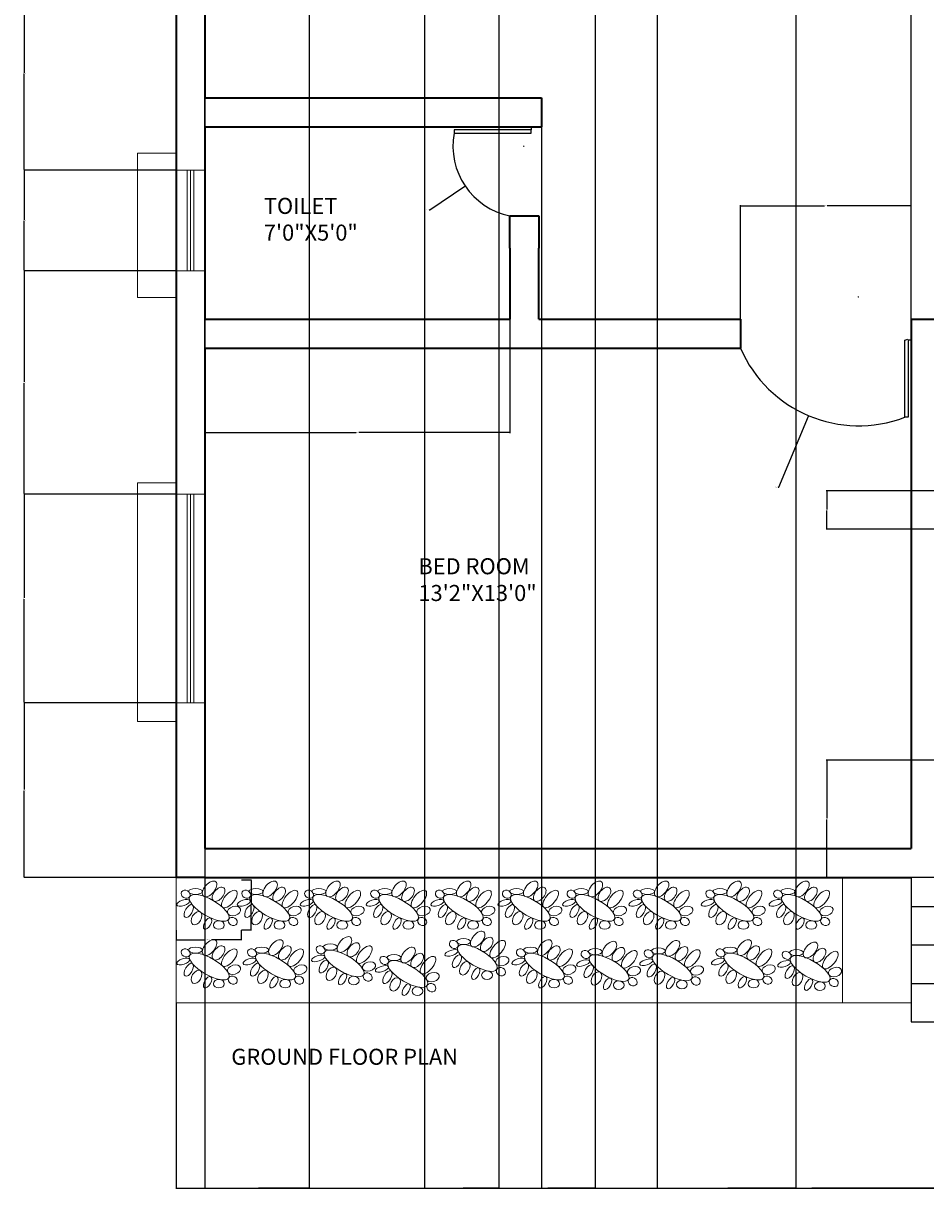
# Model space of a CAD drawing. Units: inches. Extents: x -35 to 633, y -653 to 119.
# Tile 1 of 4: x -35 to 246, y -653 to -289. Entities that reach past the tile are written whole.
import ezdxf

# ---------------------------------------------------------------- set-up
doc = ezdxf.new("R2010")
doc.units = ezdxf.units.IN
doc.header["$MEASUREMENT"] = 0
for name, color, linetype, lineweight in [('A-ANNO-DIMS', 2, 'Continuous', 18), ('A-ANNO-TEXT', 7, 'Continuous', 25), ('A-AREA-IDEN', 7, 'Continuous', 18), ('A-DOOR', 3, 'Continuous', 25), ('A-FLOR-STRS', 7, 'Continuous', 25), ('A-GLAZ', 4, 'Continuous', 20), ('A-GLAZ-PROJ', 4, 'Continuous', 18), ('A-WALL', 7, 'Continuous', 35), ('L-PLNT', 3, 'Continuous', 13), ('L-PLNT-BEDS', 94, 'Continuous', 20)]:
    doc.layers.add(name, color=color, linetype=linetype, lineweight=lineweight)
doc.styles.get("Standard").update_dxf_attribs({"font": 'arial.ttf'})
doc.dimstyles.get("Standard").update_dxf_attribs({"dimtxt": 0.18, "dimasz": 0.18, "dimexe": 0.18, "dimexo": 0.0625, "dimgap": 0.09, "dimtad": 0, "dimtih": 1, "dimtoh": 1, "dimdec": 4, "dimzin": 0, "dimdsep": 46, "dimtxsty": 'Standard', "dimcen": 0.09, "dimadec": 0, "dimazin": 0, "dimtfac": 1, "dimtdec": 4, "dimtofl": 0, "dimtmove": 0, "dimatfit": 3, "dimfxl": 1, "dimtolj": 1, "dimtzin": 0, "dimarcsym": 0})

# ---------------------------------------------------------------- blocks, each defined once
blk = doc.blocks.new('SHRUB-PLAN')
for centre, major_axis, ratio in [((0.11, 5.9), (-1.92, -2.24), 0.535049), ((-7.34, 4.24), (1.26, -0.73), 0.824136), ((0, 0), (-6.08, 3.51), 0.369459), ((-4.3, 5.11), (2.15, 0), 0.440675), ((2.91, 4.24), (-1.61, -2), 0.581787), ((6.3, 2.75), (-2.14, -2.56), 0.458164), ((-8.09, 1.57), (2.03, 0.66), 0.398765), ((-6.37, -0.99), (1.12, 1.93), 0.488989), ((7.75, -0.97), (-2.05, -0.58), 0.66194), ((-3.94, -3.23), (1.13, 1.96), 0.622261), ((-0.49, -4.89), (1, 1.73), 0.484407), ((7.35, -4.24), (-1.27, 0.73), 0.849112), ((3.02, -5.34), (-1.69, 0), 0.789987)]:
    blk.add_ellipse(centre, major_axis=major_axis, ratio=ratio)
blk = doc.blocks.new('DOOR-LEAF-24IN')
for p, q in [((-1, 24), (-2, 24)), ((-2, 24), (-2, 0)), ((-1, 0), (-1, 24)), ((-2, 0), (-1, 0)), ((0, 0), (-1, 0))]:
    blk.add_line(p, q)
blk = doc.blocks.new('*D8')
at = {"layer": 'A-ANNO-DIMS', "color": 0, "lineweight": -2, "transparency": 16777216}
for p, q in [((12.74, -572.14), (12.74, -575.29)), ((33.02, -572.14), (33.02, -575.29)), ((12.92, -575.11), (21.88, -575.11)), ((32.84, -575.11), (23.88, -575.11))]:
    blk.add_line(p, q, dxfattribs=at)
at = {"layer": 'A-ANNO-DIMS', "color": 0, "transparency": 16777216}
for points in [[(12.92, -575.08), (12.92, -575.14), (12.74, -575.11)], [(32.84, -575.08), (32.84, -575.14), (33.02, -575.11)]]:
    blk.add_solid(points, dxfattribs=at)
at = {"layer": 'Defpoints', "color": 0, "transparency": 16777216}
for p in [(12.74, -572.07), (33.02, -572.07), (33.02, -575.11)]:
    blk.add_point(p, dxfattribs=at)
at = {"layer": 'A-ANNO-DIMS', "color": 0, "transparency": 16777216, "insert": (22.88, -575.11), "char_height": 0.18, "attachment_point": 5}
blk.add_mtext('\\A1;SHRUB 20 TYP.', dxfattribs=at)
blk = doc.blocks.new('*D9')
at = {"layer": 'A-ANNO-DIMS', "color": 0, "lineweight": -2, "transparency": 16777216}
for p, q in [((33.08, -556.48), (36.24, -556.48)), ((36.06, -556.66), (36.06, -564.09)), ((36.06, -571.89), (36.06, -564.46)), ((33.08, -572.07), (36.24, -572.07))]:
    blk.add_line(p, q, dxfattribs=at)
at = {"layer": 'A-ANNO-DIMS', "color": 0, "transparency": 16777216}
for points in [[(36.03, -556.66), (36.09, -556.66), (36.06, -556.48)], [(36.03, -571.89), (36.09, -571.89), (36.06, -572.07)]]:
    blk.add_solid(points, dxfattribs=at)
at = {"layer": 'Defpoints', "color": 0, "transparency": 16777216}
for p in [(33.02, -556.48), (36.06, -556.48), (33.02, -572.07)]:
    blk.add_point(p, dxfattribs=at)
at = {"layer": 'A-ANNO-DIMS', "color": 0, "transparency": 16777216, "insert": (36.06, -564.28), "char_height": 0.18, "attachment_point": 5}
blk.add_mtext('\\A1;16 TYP.', dxfattribs=at)
blk = doc.blocks.new('*D10')
at = {"layer": 'A-ANNO-DIMS', "color": 0, "lineweight": -2, "transparency": 16777216}
for p, q in [((12.69, -594.87), (12.69, -652.72)), ((585.69, -595.88), (585.69, -652.72)), ((12.87, -652.54), (298.9, -652.54)), ((585.51, -652.54), (299.48, -652.54))]:
    blk.add_line(p, q, dxfattribs=at)
at = {"layer": 'A-ANNO-DIMS', "color": 0, "transparency": 16777216}
for points in [[(12.87, -652.51), (12.87, -652.57), (12.69, -652.54)], [(585.51, -652.51), (585.51, -652.57), (585.69, -652.54)]]:
    blk.add_solid(points, dxfattribs=at)
at = {"layer": 'Defpoints', "color": 0, "transparency": 16777216}
for p in [(12.69, -594.81), (585.69, -595.82), (585.69, -652.54)]:
    blk.add_point(p, dxfattribs=at)
at = {"layer": 'A-ANNO-DIMS', "color": 0, "transparency": 16777216, "insert": (299.19, -652.54), "char_height": 0.18, "attachment_point": 5}
blk.add_mtext('\\A1;573', dxfattribs=at)
blk = doc.blocks.new('*D14')
at = {"layer": 'A-ANNO-DIMS', "color": 0, "lineweight": -2, "transparency": 16777216}
for p, q in [((21.69, 17.22), (21.69, -652.72)), ((54.19, 17.22), (54.19, -652.72)), ((21.87, -652.54), (37.47, -652.54)), ((54.01, -652.54), (38.4, -652.54))]:
    blk.add_line(p, q, dxfattribs=at)
at = {"layer": 'A-ANNO-DIMS', "color": 0, "transparency": 16777216}
for points in [[(21.87, -652.51), (21.87, -652.57), (21.69, -652.54)], [(54.01, -652.51), (54.01, -652.57), (54.19, -652.54)]]:
    blk.add_solid(points, dxfattribs=at)
at = {"layer": 'Defpoints', "color": 0, "transparency": 16777216}
for p in [(21.69, 17.29), (54.19, 17.29), (54.19, -652.54)]:
    blk.add_point(p, dxfattribs=at)
at = {"layer": 'A-ANNO-DIMS', "color": 0, "transparency": 16777216, "insert": (37.94, -652.54), "char_height": 0.18, "attachment_point": 5}
blk.add_mtext('\\A1;32.496', dxfattribs=at)
blk = doc.blocks.new('*D15')
at = {"layer": 'A-ANNO-DIMS', "color": 0, "lineweight": -2, "transparency": 16777216}
for p, q in [((90.19, 17.22), (90.19, -652.72)), ((113.38, 17.22), (113.38, -652.72)), ((90.37, -652.54), (101.32, -652.54)), ((113.2, -652.54), (102.25, -652.54))]:
    blk.add_line(p, q, dxfattribs=at)
at = {"layer": 'A-ANNO-DIMS', "color": 0, "transparency": 16777216}
for points in [[(90.37, -652.51), (90.37, -652.57), (90.19, -652.54)], [(113.2, -652.51), (113.2, -652.57), (113.38, -652.54)]]:
    blk.add_solid(points, dxfattribs=at)
at = {"layer": 'Defpoints', "color": 0, "transparency": 16777216}
for p in [(90.19, 17.29), (113.38, 17.29), (113.38, -652.54)]:
    blk.add_point(p, dxfattribs=at)
at = {"layer": 'A-ANNO-DIMS', "color": 0, "transparency": 16777216, "insert": (101.78, -652.54), "char_height": 0.18, "attachment_point": 5}
blk.add_mtext('\\A1;23.194', dxfattribs=at)
blk = doc.blocks.new('*D16')
at = {"layer": 'A-ANNO-DIMS', "color": 0, "lineweight": -2, "transparency": 16777216}
for p, q in [((113.38, 17.22), (113.38, -652.72)), ((143.38, 17.22), (143.38, -652.72)), ((113.56, -652.54), (128.16, -652.54)), ((143.2, -652.54), (128.6, -652.54))]:
    blk.add_line(p, q, dxfattribs=at)
at = {"layer": 'A-ANNO-DIMS', "color": 0, "transparency": 16777216}
for points in [[(113.56, -652.51), (113.56, -652.57), (113.38, -652.54)], [(143.2, -652.51), (143.2, -652.57), (143.38, -652.54)]]:
    blk.add_solid(points, dxfattribs=at)
at = {"layer": 'Defpoints', "color": 0, "transparency": 16777216}
for p in [(113.38, 17.29), (143.38, 17.29), (143.38, -652.54)]:
    blk.add_point(p, dxfattribs=at)
at = {"layer": 'A-ANNO-DIMS', "color": 0, "transparency": 16777216, "insert": (128.38, -652.54), "char_height": 0.18, "attachment_point": 5}
blk.add_mtext('\\A1;30', dxfattribs=at)
blk = doc.blocks.new('*D17')
at = {"layer": 'A-ANNO-DIMS', "color": 0, "lineweight": -2, "transparency": 16777216}
for p, q in [((162.69, 17.22), (162.69, -652.72)), ((205.96, 17.22), (205.96, -652.72)), ((162.87, -652.54), (183.93, -652.54)), ((205.78, -652.54), (184.72, -652.54))]:
    blk.add_line(p, q, dxfattribs=at)
at = {"layer": 'A-ANNO-DIMS', "color": 0, "transparency": 16777216}
for points in [[(162.87, -652.51), (162.87, -652.57), (162.69, -652.54)], [(205.78, -652.51), (205.78, -652.57), (205.96, -652.54)]]:
    blk.add_solid(points, dxfattribs=at)
at = {"layer": 'Defpoints', "color": 0, "transparency": 16777216}
for p in [(162.69, 17.29), (205.96, 17.29), (205.96, -652.54)]:
    blk.add_point(p, dxfattribs=at)
at = {"layer": 'A-ANNO-DIMS', "color": 0, "transparency": 16777216, "insert": (184.33, -652.54), "char_height": 0.18, "attachment_point": 5}
blk.add_mtext('\\A1;43.27', dxfattribs=at)
blk = doc.blocks.new('*D31')
at = {"layer": 'A-ANNO-DIMS', "color": 0, "lineweight": -2, "transparency": 16777216}
for p, q in [((12.63, -274.96), (-34.84, -274.96)), ((-34.66, -275.14), (-34.66, -304.9)), ((-34.66, -335.03), (-34.66, -305.27)), ((12.63, -335.21), (-34.84, -335.21))]:
    blk.add_line(p, q, dxfattribs=at)
at = {"layer": 'A-ANNO-DIMS', "color": 0, "transparency": 16777216}
for points in [[(-34.69, -275.14), (-34.63, -275.14), (-34.66, -274.96)], [(-34.69, -335.03), (-34.63, -335.03), (-34.66, -335.21)]]:
    blk.add_solid(points, dxfattribs=at)
at = {"layer": 'Defpoints', "color": 0, "transparency": 16777216}
for p in [(12.69, -274.96), (-34.66, -335.21), (12.69, -335.21)]:
    blk.add_point(p, dxfattribs=at)
at = {"layer": 'A-ANNO-DIMS', "color": 0, "transparency": 16777216, "insert": (-34.66, -305.09), "char_height": 0.18, "attachment_point": 5}
blk.add_mtext('\\A1;60.25', dxfattribs=at)
blk = doc.blocks.new('*D32')
at = {"layer": 'A-ANNO-DIMS', "color": 0, "lineweight": -2, "transparency": 16777216}
for p, q in [((12.63, -335.21), (-34.84, -335.21)), ((-34.66, -335.39), (-34.66, -350.72)), ((-34.66, -366.41), (-34.66, -351.09)), ((12.63, -366.59), (-34.84, -366.59))]:
    blk.add_line(p, q, dxfattribs=at)
at = {"layer": 'A-ANNO-DIMS', "color": 0, "transparency": 16777216}
for points in [[(-34.69, -335.39), (-34.63, -335.39), (-34.66, -335.21)], [(-34.69, -366.41), (-34.63, -366.41), (-34.66, -366.59)]]:
    blk.add_solid(points, dxfattribs=at)
at = {"layer": 'Defpoints', "color": 0, "transparency": 16777216}
for p in [(12.69, -335.21), (-34.66, -366.59), (12.69, -366.59)]:
    blk.add_point(p, dxfattribs=at)
at = {"layer": 'A-ANNO-DIMS', "color": 0, "transparency": 16777216, "insert": (-34.66, -350.9), "char_height": 0.18, "attachment_point": 5}
blk.add_mtext('\\A1;31.38', dxfattribs=at)
blk = doc.blocks.new('*D33')
at = {"layer": 'A-ANNO-DIMS', "color": 0, "lineweight": -2, "transparency": 16777216}
for p, q in [((12.63, -366.59), (-34.84, -366.59)), ((-34.66, -366.77), (-34.66, -401.24)), ((-34.66, -436.06), (-34.66, -401.6)), ((12.63, -436.24), (-34.84, -436.24))]:
    blk.add_line(p, q, dxfattribs=at)
at = {"layer": 'A-ANNO-DIMS', "color": 0, "transparency": 16777216}
for points in [[(-34.69, -366.77), (-34.63, -366.77), (-34.66, -366.59)], [(-34.69, -436.06), (-34.63, -436.06), (-34.66, -436.24)]]:
    blk.add_solid(points, dxfattribs=at)
at = {"layer": 'Defpoints', "color": 0, "transparency": 16777216}
for p in [(12.69, -366.59), (-34.66, -436.24), (12.69, -436.24)]:
    blk.add_point(p, dxfattribs=at)
at = {"layer": 'A-ANNO-DIMS', "color": 0, "transparency": 16777216, "insert": (-34.66, -401.42), "char_height": 0.18, "attachment_point": 5}
blk.add_mtext('\\A1;69.65', dxfattribs=at)
blk = doc.blocks.new('*D34')
at = {"layer": 'A-ANNO-DIMS', "color": 0, "lineweight": -2, "transparency": 16777216}
for p, q in [((12.63, -436.24), (-34.84, -436.24)), ((-34.66, -436.42), (-34.66, -468.57)), ((-34.66, -501.09), (-34.66, -468.94)), ((12.63, -501.27), (-34.84, -501.27))]:
    blk.add_line(p, q, dxfattribs=at)
at = {"layer": 'A-ANNO-DIMS', "color": 0, "transparency": 16777216}
for points in [[(-34.69, -436.42), (-34.63, -436.42), (-34.66, -436.24)], [(-34.69, -501.09), (-34.63, -501.09), (-34.66, -501.27)]]:
    blk.add_solid(points, dxfattribs=at)
at = {"layer": 'Defpoints', "color": 0, "transparency": 16777216}
for p in [(12.69, -436.24), (-34.66, -501.27), (12.69, -501.27)]:
    blk.add_point(p, dxfattribs=at)
at = {"layer": 'A-ANNO-DIMS', "color": 0, "transparency": 16777216, "insert": (-34.66, -468.76), "char_height": 0.18, "attachment_point": 5}
blk.add_mtext('\\A1;65.02', dxfattribs=at)
blk = doc.blocks.new('*D35')
at = {"layer": 'A-ANNO-DIMS', "color": 0, "lineweight": -2, "transparency": 16777216}
for p, q in [((12.63, -501.27), (-34.84, -501.27)), ((-34.66, -501.45), (-34.66, -528.31)), ((-34.66, -555.53), (-34.66, -528.67)), ((12.63, -555.71), (-34.84, -555.71))]:
    blk.add_line(p, q, dxfattribs=at)
at = {"layer": 'A-ANNO-DIMS', "color": 0, "transparency": 16777216}
for points in [[(-34.69, -501.45), (-34.63, -501.45), (-34.66, -501.27)], [(-34.69, -555.53), (-34.63, -555.53), (-34.66, -555.71)]]:
    blk.add_solid(points, dxfattribs=at)
at = {"layer": 'Defpoints', "color": 0, "transparency": 16777216}
for p in [(12.69, -501.27), (-34.66, -555.71), (12.69, -555.71)]:
    blk.add_point(p, dxfattribs=at)
at = {"layer": 'A-ANNO-DIMS', "color": 0, "transparency": 16777216, "insert": (-34.66, -528.49), "char_height": 0.18, "attachment_point": 5}
blk.add_mtext('\\A1;54.45', dxfattribs=at)
blk = doc.blocks.new('*D36')
at = {"layer": 'A-ANNO-DIMS', "color": 0, "lineweight": -2, "transparency": 16777216}
for p, q in [((21.69, -546.65), (21.69, 118.82)), ((21.87, 118.64), (131.44, 118.64)), ((241.8, 118.64), (132.23, 118.64)), ((241.98, -546.65), (241.98, 118.82))]:
    blk.add_line(p, q, dxfattribs=at)
at = {"layer": 'A-ANNO-DIMS', "color": 0, "transparency": 16777216}
for points in [[(21.87, 118.67), (21.87, 118.61), (21.69, 118.64)], [(241.8, 118.67), (241.8, 118.61), (241.98, 118.64)]]:
    blk.add_solid(points, dxfattribs=at)
at = {"layer": 'Defpoints', "color": 0, "transparency": 16777216}
for p in [(241.98, 118.64), (21.69, -546.71), (241.98, -546.71)]:
    blk.add_point(p, dxfattribs=at)
at = {"layer": 'A-ANNO-DIMS', "color": 0, "transparency": 16777216, "insert": (131.83, 118.64), "char_height": 0.18, "attachment_point": 5}
blk.add_mtext('\\A1;220.3', dxfattribs=at)
blk = doc.blocks.new('*D39')
at = {"layer": 'A-ANNO-DIMS', "color": 0, "lineweight": -2, "transparency": 16777216}
for p, q in [((21.69, -381.78), (21.69, -417.24)), ((116.82, -381.78), (116.82, -417.24)), ((21.87, -417.06), (68.86, -417.06)), ((116.64, -417.06), (69.65, -417.06))]:
    blk.add_line(p, q, dxfattribs=at)
at = {"layer": 'A-ANNO-DIMS', "color": 0, "transparency": 16777216}
for points in [[(21.87, -417.03), (21.87, -417.09), (21.69, -417.06)], [(116.64, -417.03), (116.64, -417.09), (116.82, -417.06)]]:
    blk.add_solid(points, dxfattribs=at)
at = {"layer": 'Defpoints', "color": 0, "transparency": 16777216}
for p in [(21.69, -381.71), (116.82, -381.71), (21.69, -417.06)]:
    blk.add_point(p, dxfattribs=at)
at = {"layer": 'A-ANNO-DIMS', "color": 0, "transparency": 16777216, "insert": (69.26, -417.06), "char_height": 0.18, "attachment_point": 5}
blk.add_mtext('\\A1;95.13', dxfattribs=at)
blk = doc.blocks.new('*D42')
at = {"layer": 'A-ANNO-DIMS', "color": 0, "lineweight": -2, "transparency": 16777216}
for p, q in [((250.91, -435.17), (215.45, -435.17)), ((215.63, -435.35), (215.63, -440.99)), ((215.63, -446.99), (215.63, -441.35)), ((250.91, -447.17), (215.45, -447.17))]:
    blk.add_line(p, q, dxfattribs=at)
at = {"layer": 'A-ANNO-DIMS', "color": 0, "transparency": 16777216}
for points in [[(215.6, -435.35), (215.66, -435.35), (215.63, -435.17)], [(215.6, -446.99), (215.66, -446.99), (215.63, -447.17)]]:
    blk.add_solid(points, dxfattribs=at)
at = {"layer": 'Defpoints', "color": 0, "transparency": 16777216}
for p in [(215.63, -435.17), (250.98, -435.17), (250.98, -447.17)]:
    blk.add_point(p, dxfattribs=at)
at = {"layer": 'A-ANNO-DIMS', "color": 0, "transparency": 16777216, "insert": (215.63, -441.17), "char_height": 0.18, "attachment_point": 5}
blk.add_mtext('\\A1;12', dxfattribs=at)
blk = doc.blocks.new('*D43')
at = {"layer": 'A-ANNO-DIMS', "color": 0, "lineweight": -2, "transparency": 16777216}
for p, q in [((250.91, -519.17), (215.45, -519.17)), ((215.63, -519.35), (215.63, -537.26)), ((215.63, -555.53), (215.63, -537.62)), ((250.91, -555.71), (215.45, -555.71))]:
    blk.add_line(p, q, dxfattribs=at)
at = {"layer": 'A-ANNO-DIMS', "color": 0, "transparency": 16777216}
for points in [[(215.6, -519.35), (215.66, -519.35), (215.63, -519.17)], [(215.6, -555.53), (215.66, -555.53), (215.63, -555.71)]]:
    blk.add_solid(points, dxfattribs=at)
at = {"layer": 'Defpoints', "color": 0, "transparency": 16777216}
for p in [(215.63, -519.17), (250.98, -519.17), (250.98, -555.71)]:
    blk.add_point(p, dxfattribs=at)
at = {"layer": 'A-ANNO-DIMS', "color": 0, "transparency": 16777216, "insert": (215.63, -537.44), "char_height": 0.18, "attachment_point": 5}
blk.add_mtext('\\A1;36.54', dxfattribs=at)
blk = doc.blocks.new('*D45')
at = {"layer": 'A-ANNO-DIMS', "color": 0, "lineweight": -2, "transparency": 16777216}
for p, q in [((188.69, -381.65), (188.69, -346.18)), ((188.87, -346.36), (214.94, -346.36)), ((241.8, -346.36), (215.73, -346.36)), ((241.98, -381.65), (241.98, -346.18))]:
    blk.add_line(p, q, dxfattribs=at)
at = {"layer": 'A-ANNO-DIMS', "color": 0, "transparency": 16777216}
for points in [[(188.87, -346.33), (188.87, -346.39), (188.69, -346.36)], [(241.8, -346.33), (241.8, -346.39), (241.98, -346.36)]]:
    blk.add_solid(points, dxfattribs=at)
at = {"layer": 'Defpoints', "color": 0, "transparency": 16777216}
for p in [(241.98, -346.36), (188.69, -381.71), (241.98, -381.71)]:
    blk.add_point(p, dxfattribs=at)
at = {"layer": 'A-ANNO-DIMS', "color": 0, "transparency": 16777216, "insert": (215.33, -346.36), "char_height": 0.18, "attachment_point": 5}
blk.add_mtext('\\A1;53.29', dxfattribs=at)
blk = doc.blocks.new('*D47')
at = {"layer": 'A-ANNO-DIMS', "color": 0, "lineweight": -2, "transparency": 16777216}
for p, q in [((294.69, -123.78), (294.69, -652.72)), ((126.69, -312.78), (126.69, -652.72)), ((126.87, -652.54), (210.41, -652.54)), ((294.51, -652.54), (210.97, -652.54))]:
    blk.add_line(p, q, dxfattribs=at)
at = {"layer": 'A-ANNO-DIMS', "color": 0, "transparency": 16777216}
for points in [[(126.87, -652.51), (126.87, -652.57), (126.69, -652.54)], [(294.51, -652.51), (294.51, -652.57), (294.69, -652.54)]]:
    blk.add_solid(points, dxfattribs=at)
at = {"layer": 'Defpoints', "color": 0, "transparency": 16777216}
for p in [(294.69, -123.71), (126.69, -312.71), (294.69, -652.54)]:
    blk.add_point(p, dxfattribs=at)
at = {"layer": 'A-ANNO-DIMS', "color": 0, "transparency": 16777216, "insert": (210.69, -652.54), "char_height": 0.18, "attachment_point": 5}
blk.add_mtext('\\A1;168', dxfattribs=at)
blk = doc.blocks.new('*D49')
at = {"layer": 'A-ANNO-DIMS', "color": 0, "lineweight": -2, "transparency": 16777216}
for p, q in [((225.47, -374.75), (225.65, -374.75)), ((225.56, -374.84), (225.56, -374.66)), ((200.67, -434.02), (209.93, -411.96)), ((200.49, -434.02), (200.67, -434.02))]:
    blk.add_line(p, q, dxfattribs=at)
at = {"layer": 'A-ANNO-DIMS', "color": 0, "transparency": 16777216}
blk.add_solid([(209.91, -411.95), (209.96, -411.97), (210, -411.79)], dxfattribs=at)
at = {"layer": 'Defpoints', "color": 0, "transparency": 16777216}
for p in [(225.56, -374.75), (210, -411.79)]:
    blk.add_point(p, dxfattribs=at)
at = {"layer": 'A-ANNO-DIMS', "color": 0, "transparency": 16777216, "insert": (200.01, -434.02), "char_height": 0.18, "attachment_point": 5}
blk.add_mtext('\\A1;R40.18', dxfattribs=at)
blk = doc.blocks.new('*D62')
at = {"layer": 'A-ANNO-DIMS', "color": 0, "lineweight": -2, "transparency": 16777216}
for p, q in [((121.1, -327.79), (121.28, -327.79)), ((121.19, -327.88), (121.19, -327.7)), ((91.83, -347.6), (102.69, -340.27)), ((91.65, -347.6), (91.83, -347.6))]:
    blk.add_line(p, q, dxfattribs=at)
at = {"layer": 'A-ANNO-DIMS', "color": 0, "transparency": 16777216}
blk.add_solid([(102.67, -340.25), (102.7, -340.3), (102.84, -340.17)], dxfattribs=at)
at = {"layer": 'Defpoints', "color": 0, "transparency": 16777216}
for p in [(121.19, -327.79), (102.84, -340.17)]:
    blk.add_point(p, dxfattribs=at)
at = {"layer": 'A-ANNO-DIMS', "color": 0, "transparency": 16777216, "insert": (91.17, -347.6), "char_height": 0.18, "attachment_point": 5}
blk.add_mtext('\\A1;R22.14', dxfattribs=at)

msp = doc.modelspace()

# ---------------------------------------------------------------- linework, layer by layer
at = {"layer": 'A-DOOR'}
for p, q in [((239.9768, -388.2565), (240.93, -387.9542)), ((239.9768, -412.2565), (239.9768, -388.2565)), ((241.9768, -388.2565), (240.9768, -388.2565)), ((240.9768, -388.2565), (240.9768, -412.2565)), ((240.9768, -412.2565), (239.9768, -412.2565))]:
    msp.add_line(p, q, dxfattribs=at)
for centre, radius, start, end in [((121.1872, -327.787), 22.14, 169.396444, 258.635476), ((225.564, -374.7501), 40.1803, 203.408275, 291.02059)]:
    msp.add_arc(centre, radius, start, end, dxfattribs=at)
at = {"layer": 'A-FLOR-STRS'}
for p, q in [((241.9768, -555.713), (241.9768, -564.713)), ((241.9768, -564.713), (355.9768, -564.713)), ((241.9768, -564.713), (241.9768, -600.713)), ((241.9768, -576.713), (355.9768, -576.713)), ((241.9768, -588.713), (355.9768, -588.713)), ((241.9768, -600.713), (355.9768, -600.713))]:
    msp.add_line(p, q, dxfattribs=at)
at = {"layer": 'A-GLAZ'}
for p, q in [((12.6907, -335.213), (21.6907, -335.213)), ((16.1907, -335.213), (16.1907, -366.5948)), ((17.1907, -335.213), (17.1907, -366.5948)), ((18.1907, -335.213), (18.1907, -366.5948)), ((12.6907, -366.5948), (21.6907, -366.5948)), ((12.6907, -436.2449), (21.6907, -436.2449)), ((16.1907, -436.2449), (16.1907, -501.2675)), ((17.1907, -436.2449), (17.1907, -501.2675)), ((18.1907, -436.2449), (18.1907, -501.2675)), ((12.6907, -501.2675), (21.6907, -501.2675))]:
    msp.add_line(p, q, dxfattribs=at)
at = {"layer": 'A-GLAZ-PROJ'}
for p, q in [((12.6907, -329.9325), (0.6907, -329.9325)), ((0.6907, -329.9325), (0.6907, -374.8863)), ((0.6907, -374.8863), (12.6907, -374.8863)), ((12.6907, -432.7076), (0.6907, -432.7076)), ((0.6907, -432.7076), (0.6907, -507.0574)), ((0.6907, -507.0574), (12.6907, -507.0574))]:
    msp.add_line(p, q, dxfattribs=at)
at = {"layer": 'A-WALL'}
for p, q in [((12.6907, -114.713), (12.6907, -555.713)), ((21.6907, -180.713), (21.6907, -312.713)), ((21.6907, -312.713), (114.6907, -312.713)), ((114.6907, -312.713), (126.6907, -312.713)), ((126.6907, -312.713), (126.6907, -321.713)), ((21.6907, -321.713), (114.6907, -321.713)), ((21.6907, -321.713), (21.6907, -381.713)), ((114.6907, -321.713), (126.6907, -321.713)), ((116.8245, -359.5652), (116.8245, -349.4929)), ((116.8245, -349.4929), (125.8245, -349.4929)), ((125.8245, -349.4929), (125.8245, -359.5652)), ((116.8245, -359.5652), (116.8245, -381.713)), ((125.8245, -381.713), (125.8245, -359.5652)), ((21.6907, -381.713), (114.6907, -381.713)), ((114.6907, -381.713), (116.8245, -381.713)), ((125.8245, -381.713), (188.6907, -381.713)), ((188.6907, -381.713), (188.6907, -390.713)), ((241.9768, -381.713), (250.9768, -381.713)), ((241.9768, -381.713), (241.9768, -546.713)), ((21.6907, -390.713), (114.6907, -390.713)), ((21.6907, -390.713), (21.6907, -546.713)), ((114.6907, -390.713), (188.6907, -390.713)), ((21.6907, -546.713), (114.6907, -546.713)), ((114.6907, -546.713), (188.6907, -546.713)), ((188.6907, -546.713), (241.9768, -546.713)), ((21.6907, -555.713), (12.6907, -555.713)), ((21.6907, -555.713), (114.6907, -555.713)), ((114.6907, -555.713), (188.6907, -555.713)), ((188.6907, -555.713), (241.9768, -555.713))]:
    msp.add_line(p, q, dxfattribs=at)
at = {"layer": 'L-PLNT-BEDS'}
for p, q in [((12.6907, -594.812), (12.6907, -555.713)), ((220.528, -555.713), (220.528, -594.812)), ((241.9768, -594.812), (12.6907, -594.812))]:
    msp.add_line(p, q, dxfattribs=at)

# ---------------------------------------------------------------- block references
at = {"layer": 'A-DOOR', "rotation": 90.00000000000021}
msp.add_blockref('DOOR-LEAF-24IN', (123.4252, -321.713), dxfattribs=at)
at = {"layer": 'L-PLNT'}
for p in [(23.014, -565.1885), (41.9072, -565.1885), (61.5129, -565.1885), (82.1029, -565.1885), (102.2768, -565.1885), (123.18, -565.1885), (143.3539, -565.1885), (164.014, -565.1885), (186.6185, -565.1885), (207.7647, -565.1885), (65.0887, -582.5018), (106.6519, -580.8023), (23.014, -583.4729), (43.6995, -583.4729), (84.953, -585.7934), (127.555, -583.4729), (147.729, -583.9584), (167.4168, -583.7156), (189.7783, -583.4729), (210.4383, -584.22)]:
    msp.add_blockref('SHRUB-PLAN', p, dxfattribs=at)

# ---------------------------------------------------------------- texts
at = {"layer": 'A-ANNO-TEXT', "insert": (29.8973, -609.0996), "char_height": 5, "attachment_point": 1}
msp.add_mtext_dynamic_manual_height_columns('GROUND FLOOR PLAN', width=222.508853, gutter_width=25, heights=[0], dxfattribs=at)
at = {"layer": 'A-AREA-IDEN', "char_height": 5, "attachment_point": 1}
for s, width, insert in [('TOILET\\P7\'0"X5\'0"', 31.01588, (40.0556, -343.8811)), ('BED ROOM\\P13\'2"X13\'0"', 82.004443, (88.2528, -456.2031))]:
    msp.add_mtext_dynamic_manual_height_columns(s, width=width, gutter_width=25, heights=[0], dxfattribs=dict(at, insert=insert))

# ---------------------------------------------------------------- dimensions: what is measured, and where the dimension line sits
at = {"layer": 'A-ANNO-DIMS'}
for base, p1, p2, override, picture, middle in [((241.9768, 118.637), (21.6907, -546.713), (241.9768, -546.713), {"dimdec": 1, "dimlfac": 1, "dimrnd": 0, "dimzin": 0, "dimdsep": 46, "dimlunit": 2}, '*D36', (131.8337, 118.637)), ((54.18621, -652.537), (21.69066, 17.28704), (54.18621, 17.28704), {"dimdec": 3, "dimlfac": 1, "dimrnd": 0, "dimzin": 0, "dimdsep": 46, "dimlunit": 2}, '*D14', (37.93843, -652.537)), ((113.3804, -652.537), (90.1862, 17.287), (113.3804, 17.287), {"dimdec": 3, "dimlfac": 1, "dimrnd": 0, "dimzin": 0, "dimdsep": 46, "dimlunit": 2}, '*D15', (101.7833, -652.537)), ((143.3804, -652.537), (113.3804, 17.287), (143.3804, 17.287), {"dimdec": 0, "dimlfac": 1, "dimrnd": 0, "dimzin": 0, "dimdsep": 46, "dimlunit": 2}, '*D16', (128.3804, -652.537)), ((205.9605, -652.537), (162.6907, 17.287), (205.9605, 17.287), {"dimdec": 2, "dimlfac": 1, "dimrnd": 0, "dimzin": 0, "dimdsep": 46, "dimlunit": 2}, '*D17', (184.3256, -652.537)), ((294.6907, -652.537), (126.6907, -312.713), (294.6907, -123.713), {"dimdec": 0, "dimlfac": 1, "dimrnd": 0, "dimzin": 0, "dimdsep": 46, "dimlunit": 2}, '*D47', (210.6907, -652.537)), ((241.9768, -346.363), (188.6907, -381.713), (241.9768, -381.713), {"dimdec": 2, "dimlfac": 1, "dimrnd": 0, "dimzin": 0, "dimdsep": 46, "dimlunit": 2}, '*D45', (215.3337, -346.363)), ((585.6907, -652.537), (12.6907, -594.812), (585.6907, -595.8152), {"dimdec": 0, "dimlfac": 1, "dimrnd": 0, "dimzin": 0, "dimdsep": 46, "dimlunit": 2}, '*D10', (299.1907, -652.537))]:
    dim = msp.add_linear_dim(base=base, p1=p1, p2=p2, dimstyle='Standard', override=override, dxfattribs=at)
    dim.commit()
    dim.dimension.update_dxf_attribs({"geometry": picture, "text_midpoint": middle})
for base, p1, p2, angle, override, picture, middle in [((-34.6593, -335.213), (12.6907, -274.9586), (12.6907, -335.213), 90, {"dimdec": 2, "dimlfac": 1, "dimrnd": 0, "dimzin": 0, "dimdsep": 46, "dimlunit": 2}, '*D31', (-34.6593, -305.0858)), ((-34.6593, -366.5948), (12.6907, -335.213), (12.6907, -366.5948), 90, {"dimdec": 2, "dimlfac": 1, "dimrnd": 0, "dimzin": 0, "dimdsep": 46, "dimlunit": 2}, '*D32', (-34.6593, -350.9039)), ((-34.6593, -436.2449), (12.6907, -366.5948), (12.6907, -436.2449), 90, {"dimdec": 2, "dimlfac": 1, "dimrnd": 0, "dimzin": 0, "dimdsep": 46, "dimlunit": 2}, '*D33', (-34.6593, -401.4199)), ((21.6907, -417.063), (116.8245, -381.713), (21.6907, -381.713), 180, {"dimdec": 2, "dimlfac": 1, "dimrnd": 0, "dimzin": 0, "dimdsep": 46, "dimlunit": 2}, '*D39', (69.2576, -417.063)), ((215.6268, -435.1709), (250.9768, -447.1709), (250.9768, -435.1709), 90, {"dimdec": 0, "dimlfac": 1, "dimrnd": 0, "dimzin": 0, "dimdsep": 46, "dimlunit": 2}, '*D42', (215.6268, -441.1709)), ((-34.6593, -501.2675), (12.6907, -436.2449), (12.6907, -501.2675), 90, {"dimdec": 2, "dimlfac": 1, "dimrnd": 0, "dimzin": 0, "dimdsep": 46, "dimlunit": 2}, '*D34', (-34.6593, -468.7562)), ((-34.6593, -555.713), (12.6907, -501.2675), (12.6907, -555.713), 90, {"dimdec": 2, "dimlfac": 1, "dimrnd": 0, "dimzin": 0, "dimdsep": 46, "dimlunit": 2}, '*D35', (-34.6593, -528.4902)), ((215.6268, -519.1709), (250.9768, -555.713), (250.9768, -519.1709), 90, {"dimdec": 2, "dimlfac": 1, "dimrnd": 0, "dimzin": 0, "dimdsep": 46, "dimlunit": 2}, '*D43', (215.6268, -537.4419))]:
    dim = msp.add_linear_dim(base=base, p1=p1, p2=p2, angle=angle, dimstyle='Standard', override=override, dxfattribs=at)
    dim.commit()
    dim.dimension.update_dxf_attribs({"geometry": picture, "text_midpoint": middle})
for center, mpoint, picture, middle in [((121.1872, -327.787), (102.836, -340.173), '*D62', (91.1658, -347.6046)), ((225.564, -374.7501), (210.0031, -411.7949), '*D49', (200.0065, -434.0217))]:
    dim = msp.add_radius_dim(center=center, mpoint=mpoint, dimstyle='Standard', override={"dimdec": 2, "dimlfac": 1, "dimrnd": 0, "dimzin": 0, "dimdsep": 46, "dimlunit": 2}, dxfattribs=at)
    dim.commit()
    dim.dimension.update_dxf_attribs({"geometry": picture, "text_midpoint": middle, "dimtype": 164})
dim = msp.add_linear_dim(base=(36.062, -556.4807), p1=(33.0202, -572.0728), p2=(33.0202, -556.4807), angle=90, text='<> TYP.', dimstyle='Standard', override={"dimdec": 0, "dimlfac": 1, "dimrnd": 0, "dimzin": 0, "dimdsep": 46, "dimlunit": 2}, dxfattribs=at)
dim.commit()
dim.dimension.update_dxf_attribs({"geometry": '*D9', "text_midpoint": (36.062, -564.2768)})
dim = msp.add_linear_dim(base=(33.0202, -575.1146), p1=(12.7415, -572.0728), p2=(33.0202, -572.0728), text='SHRUB <> TYP.', dimstyle='Standard', override={"dimdec": 0, "dimlfac": 1, "dimrnd": 0, "dimzin": 0, "dimdsep": 46, "dimlunit": 2}, dxfattribs=at)
dim.commit()
dim.dimension.update_dxf_attribs({"geometry": '*D8', "text_midpoint": (22.8808, -575.1146)})

doc.saveas('drawing.dxf')
